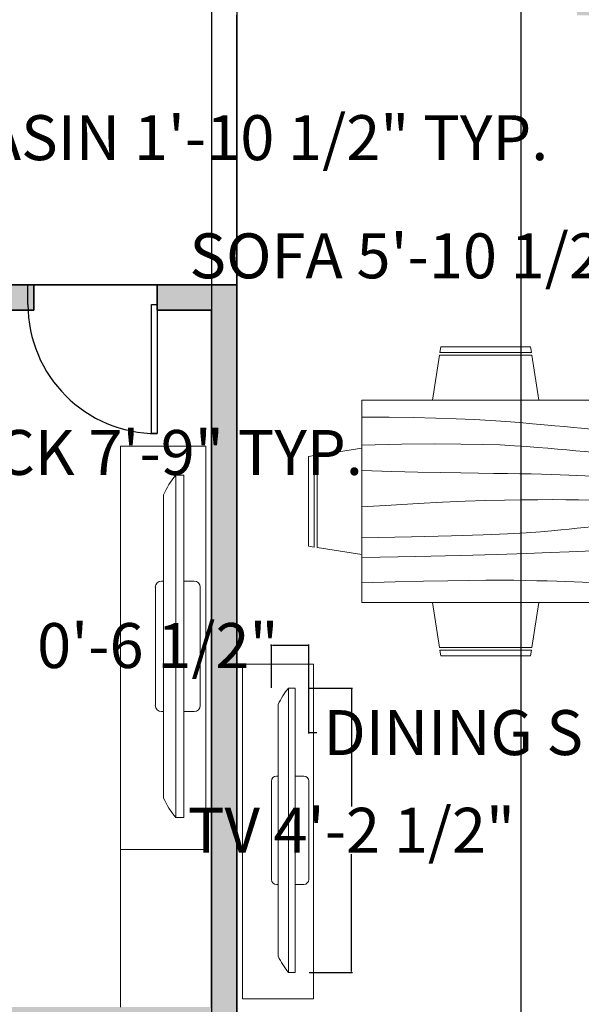
# Model space of a CAD drawing. Units: inches. Extents: x -4737294 to -4736756, y 1716389 to 1717040.
# Tile 18 of 25: x -4737096 to -4736996, y 1716669 to 1716844. Entities that reach past the tile are written whole.
import ezdxf

# ---------------------------------------------------------------- set-up
doc = ezdxf.new("R2010")
doc.units = ezdxf.units.IN
doc.header["$MEASUREMENT"] = 0
for name, color, linetype, lineweight in [('A-ANNO-DIMS', 2, 'Continuous', 18), ('A-WALL-PATT', 244, 'Continuous', 13), ('doors', 252, 'Continuous', 25), ('furniture', 250, 'Continuous', 18), ('walls', 252, 'Continuous', 35)]:
    doc.layers.add(name, color=color, linetype=linetype, lineweight=lineweight)
doc.styles.get("Standard").update_dxf_attribs({"font": 'arial.ttf'})
doc.dimstyles.get("Standard").update_dxf_attribs({"dimtxt": 8, "dimasz": 0.18, "dimexe": 0.18, "dimexo": 0.0625, "dimgap": 0.09, "dimtad": 0, "dimtih": 1, "dimtoh": 1, "dimzin": 0, "dimdsep": 46, "dimlunit": 3, "dimtxsty": 'Standard', "dimcen": 0.09, "dimadec": 0, "dimazin": 0, "dimtfac": 1, "dimtofl": 0, "dimtmove": 0, "dimatfit": 3, "dimfxl": 1, "dimtolj": 1, "dimtzin": 0, "dimarcsym": 0})

# ---------------------------------------------------------------- blocks, each defined once
blk = doc.blocks.new('Dining Set - 36 x 72 in.')
for p, q in [((-22, 27.5), (-22.1562, 26.50042)), ((-5.8416, 26.5), (-22.1534, 26.5)), ((-22, 27.5), (-6, 27.5)), ((-5.8437, 26.49966), (-6, 27.5)), ((6, 27.5), (5.8438, 26.50042)), ((22.1584, 26.5), (5.8466, 26.5)), ((6, 27.5), (22, 27.5)), ((22.1563, 26.49966), (22, 27.5)), ((-22.2343, 26.00059), (-23.4847, 17.99762)), ((-22.2304, 26), (-5.7608, 26)), ((-4.5152, 17.99762), (-5.7655, 25.99926)), ((5.7657, 26.00059), (4.5153, 17.99762)), ((5.7696, 26), (22.2392, 26)), ((23.4848, 17.99762), (22.2345, 25.99926)), ((36, 18), (-36, 18)), ((-36, 18), (-36, -18)), ((36, -18), (36, 18)), ((-44.0006, 8.23428), (-35.9976, 9.48474)), ((44.0006, 8.23428), (35.9976, 9.48474)), ((-45.5, 8), (-44.5004, 8.15617)), ((-45.5, 8), (-45.5, -8)), ((-44.5, -8.15843), (-44.5, 8.15338)), ((-44, 8.23041), (-44, -8.23915)), ((44, 8.23041), (44, -8.23915)), ((44.5, -8.15843), (44.5, 8.15338)), ((45.5, 8), (44.5005, 8.15617)), ((45.5, 8), (45.5, -8)), ((-44.4997, -8.15631), (-45.5, -8)), ((-35.9976, -9.48476), (-43.9993, -8.2345)), ((35.9976, -9.48476), (43.9993, -8.2345)), ((44.4997, -8.15631), (45.5, -8)), ((-36, -18), (36, -18)), ((-22.2343, -26.0006), (-23.4847, -17.99762)), ((-4.5152, -17.99762), (-5.7655, -25.99928)), ((5.7657, -26.0006), (4.5153, -17.99762)), ((23.4848, -17.99762), (22.2345, -25.99928)), ((-22.2304, -26), (-5.7608, -26)), ((5.7696, -26), (22.2392, -26)), ((-22, -27.5), (-22.1562, -26.50044)), ((-5.8416, -26.5), (-22.1534, -26.5)), ((-22, -27.5), (-6, -27.5)), ((-5.8437, -26.49967), (-6, -27.5)), ((6, -27.5), (5.8438, -26.50044)), ((22.1584, -26.5), (5.8466, -26.5)), ((6, -27.5), (22, -27.5)), ((22.1563, -26.49967), (22, -27.5))]:
    blk.add_line(p, q)
for points in [[(-36, 15), (-31.1772, 14.97754), (-26.8079, 14.91406), (-22.8538, 14.81543), (-19.276, 14.6875), (-16.0362, 14.53613), (-13.0957, 14.36718), (-10.4159, 14.18652), (-7.9583, 14), (-5.6904, 13.81315), (-3.6035, 13.63021), (-1.6954, 13.45508), (0.0365, 13.29166), (1.5945, 13.14388), (2.9811, 13.01562), (4.1988, 12.9108), (5.25, 12.83333), (6.1393, 12.78613), (6.8802, 12.76823), (7.4883, 12.77767), (7.9792, 12.8125), (8.3685, 12.87077), (8.6719, 12.95052), (8.9049, 13.0498), (9.0833, 13.16666), (9.2205, 13.29899), (9.3216, 13.44401), (9.3895, 13.59879), (9.4271, 13.76041), (9.4373, 13.92594), (9.4232, 14.09245), (9.3875, 14.257), (9.3333, 14.41666), (9.2638, 14.56917), (9.1836, 14.71484), (9.0975, 14.85465), (9.0104, 14.98958), (8.9272, 15.1206), (8.8529, 15.2487), (8.7922, 15.37483), (8.75, 15.5), (8.7305, 15.62467), (8.7344, 15.74739), (8.7617, 15.86621), (8.8125, 15.97916), (8.8867, 16.08431), (8.9844, 16.17968), (9.1055, 16.26334), (9.25, 16.33333), (9.4189, 16.38802), (9.6172, 16.42708), (9.8506, 16.45052), (10.125, 16.45833), (10.4463, 16.45052), (10.8203, 16.42708), (11.2529, 16.38802), (11.75, 16.33333), (12.3184, 16.26318), (12.9694, 16.17838), (13.7151, 16.07991), (14.5677, 15.96875), (15.5395, 15.84586), (16.6426, 15.71224), (17.8893, 15.56884), (19.2917, 15.41666), (20.859, 15.25667), (22.5879, 15.08984), (24.4721, 14.91715), (26.5052, 14.73958), (28.6809, 14.5581), (30.9929, 14.3737), (33.4347, 14.18733), (36, 14)], [(-36, 10), (-28.9766, 10.14274), (-23.1725, 10.20442), (-18.4241, 10.19775), (-14.5677, 10.13541), (-11.4399, 10.03011), (-8.877, 9.89453), (-6.7154, 9.74137), (-4.7917, 9.58333), (-2.9698, 9.43082), (-1.2246, 9.28515), (0.4415, 9.14534), (2.026, 9.01041), (3.5266, 8.87939), (4.9408, 8.7513), (6.266, 8.62516), (7.5, 8.5), (8.6411, 8.37549), (9.6914, 8.2539), (10.6538, 8.13818), (11.5312, 8.03125), (12.3267, 7.93603), (13.043, 7.85547), (13.6831, 7.79248), (14.25, 7.75), (14.7471, 7.7303), (15.1797, 7.73307), (15.5537, 7.75732), (15.875, 7.80208), (16.1494, 7.86637), (16.3828, 7.94922), (16.5811, 8.04964), (16.75, 8.16666), (16.8944, 8.29915), (17.0143, 8.44531), (17.1089, 8.60319), (17.1771, 8.77083), (17.218, 8.94629), (17.2305, 9.1276), (17.2137, 9.31282), (17.1667, 9.5), (17.0895, 9.6875), (16.987, 9.875), (16.8649, 10.0625), (16.7292, 10.25), (16.5856, 10.4375), (16.4401, 10.625), (16.2985, 10.8125), (16.1667, 11), (16.05, 11.18733), (15.9518, 11.3737), (15.8752, 11.5581), (15.8229, 11.73958), (15.798, 11.91715), (15.8034, 12.08984), (15.842, 12.25667), (15.9167, 12.41666), (16.0295, 12.56836), (16.1784, 12.70833), (16.3605, 12.83268), (16.5729, 12.9375), (16.8127, 13.01888), (17.0768, 13.07291), (17.3625, 13.0957), (17.6667, 13.08333), (17.9894, 13.03312), (18.3418, 12.94726), (18.7382, 12.82918), (19.1927, 12.68229), (19.7195, 12.51001), (20.3327, 12.31575), (21.0465, 12.10294), (21.875, 11.875), (22.8357, 11.63354), (23.959, 11.37304), (25.2786, 11.08618), (26.8282, 10.76562), (28.6414, 10.40405), (30.752, 9.99414), (33.1936, 9.52856), (36, 9)], [(-36, 5.5), (-30.7157, 5.3348), (-26.069, 5.20963), (-21.9946, 5.11767), (-18.4271, 5.05208), (-15.3009, 5.00602), (-12.5508, 4.97265), (-10.1112, 4.94515), (-7.9167, 4.91666), (-5.909, 4.88167), (-4.0586, 4.83984), (-2.3429, 4.79215), (-0.7396, 4.73958), (0.7739, 4.6831), (2.22, 4.6237), (3.6213, 4.56233), (5, 4.5), (6.373, 4.43782), (7.7344, 4.3776), (9.0723, 4.32129), (10.375, 4.27083), (11.6309, 4.22819), (12.8281, 4.19531), (13.9551, 4.17415), (15, 4.16666), (15.954, 4.17448), (16.819, 4.19791), (17.6001, 4.23698), (18.3021, 4.29166), (18.9299, 4.36198), (19.4883, 4.44791), (19.9823, 4.54948), (20.4167, 4.66666), (20.7969, 4.79899), (21.1302, 4.94401), (21.4245, 5.09879), (21.6875, 5.26041), (21.9271, 5.42594), (22.1511, 5.59245), (22.3672, 5.757), (22.5834, 5.91666), (22.8065, 6.06868), (23.0404, 6.21093), (23.2879, 6.34147), (23.5521, 6.45833), (23.8358, 6.55957), (24.142, 6.64323), (24.4735, 6.70735), (24.8334, 6.75), (25.2235, 6.76969), (25.642, 6.76692), (26.0858, 6.74267), (26.5521, 6.69791), (27.0379, 6.63362), (27.5404, 6.55078), (28.0565, 6.45036), (28.5834, 6.33333), (29.1242, 6.19987), (29.7071, 6.04687), (30.3661, 5.87044), (31.1354, 5.66666), (32.0493, 5.43164), (33.142, 5.16146), (34.4475, 4.85221), (36, 4.5)], [(-36, -1), (-30.7915, -0.6591), (-26.0195, -0.38216), (-21.6519, -0.16284), (-17.6563, 0.00521), (-14.0005, 0.12833), (-10.6523, 0.21289), (-7.5796, 0.26522), (-4.75, 0.29166), (-2.134, 0.29793), (0.2878, 0.28711), (2.5317, 0.26163), (4.6146, 0.22396), (6.5529, 0.17651), (8.3633, 0.12174), (10.0623, 0.06209), (11.6667, 0), (13.1899, -0.06201), (14.6341, -0.1211), (15.9982, -0.17432), (17.2813, -0.21875), (18.4823, -0.25147), (19.6003, -0.26953), (20.6343, -0.27002), (21.5834, -0.25), (22.4481, -0.20768), (23.2357, -0.14584), (23.9549, -0.06836), (24.6146, 0.02083), (25.2235, 0.11784), (25.7904, 0.21875), (26.3241, 0.31966), (26.8334, 0.41666), (27.3265, 0.50618), (27.8099, 0.58593), (28.2894, 0.65397), (28.7709, 0.70833), (29.2601, 0.74707), (29.763, 0.76823), (30.2855, 0.76985), (30.8334, 0.75), (31.4088, 0.70784), (31.9994, 0.64713), (32.589, 0.57275), (33.1615, 0.48958), (33.7008, 0.4025), (34.1908, 0.3164), (34.6153, 0.23616), (34.9584, 0.16666), (35.2099, 0.11165), (35.3848, 0.07031), (35.504, 0.04069), (35.5886, 0.02083), (35.6594, 0.00879), (35.7377, 0.0026), (35.8442, 0.00032), (36, 0)], [(-36, -6.5), (-27.1843, -6.31267), (-20.084, -6.1263), (-14.469, -5.9419), (-10.1094, -5.76042), (-6.7752, -5.58285), (-4.2363, -5.41016), (-2.2629, -5.24333), (-0.625, -5.08334), (0.8708, -4.93099), (2.2715, -4.78646), (3.5872, -4.64974), (4.8281, -4.52084), (6.0046, -4.39974), (7.127, -4.28646), (8.2053, -4.18099), (9.25, -4.08334), (10.2705, -3.99382), (11.2734, -3.91407), (12.2647, -3.84603), (13.25, -3.79167), (14.2354, -3.75293), (15.2266, -3.73177), (16.2295, -3.73015), (17.25, -3.75), (18.2912, -3.79248), (19.3451, -3.85547), (20.4009, -3.93604), (21.4479, -4.03125), (22.4754, -4.13819), (23.4727, -4.25391), (24.4289, -4.37549), (25.3334, -4.5), (26.1785, -4.62492), (26.9694, -4.74935), (27.7145, -4.87281), (28.4219, -4.99479), (29.1, -5.11483), (29.7572, -5.23242), (30.4016, -5.34709), (31.0417, -5.45834), (31.6837, -5.56437), (32.3262, -5.65821), (32.9658, -5.73153), (33.599, -5.77604), (34.2224, -5.78345), (34.8327, -5.74545), (35.4264, -5.65373), (36, -5.5)], [(-36, -10), (-26.4022, -9.81299), (-18.4675, -9.62891), (-11.9839, -9.45069), (-6.7396, -9.28125), (-2.5226, -9.12354), (0.8789, -8.98047), (3.6769, -8.85498), (6.0833, -8.75), (8.2767, -8.66765), (10.3021, -8.60677), (12.1712, -8.56543), (13.8958, -8.54167), (15.4876, -8.53353), (16.9583, -8.53907), (18.3197, -8.55632), (19.5834, -8.58334), (20.7616, -8.61841), (21.8685, -8.66081), (22.9188, -8.71004), (23.9271, -8.76563), (24.9081, -8.82707), (25.8763, -8.89388), (26.8465, -8.96558), (27.8334, -9.04167), (28.8474, -9.12118), (29.8828, -9.20117), (30.93, -9.27824), (31.9792, -9.34896), (33.0205, -9.40991), (34.0443, -9.45768), (35.0407, -9.48885), (36, -9.5)], [(-36, -14.5), (-30.0881, -14.33513), (-25.0332, -14.21224), (-20.7312, -14.12647), (-17.0781, -14.07292), (-13.97, -14.04671), (-11.3027, -14.04297), (-8.9724, -14.05681), (-6.875, -14.08334), (-4.9224, -14.11833), (-3.0905, -14.16016), (-1.3709, -14.20785), (0.2448, -14.26042), (1.7647, -14.3169), (3.1973, -14.3763), (4.5507, -14.43767), (5.8333, -14.5), (7.0554, -14.5621), (8.235, -14.62175), (9.3922, -14.67652), (10.5469, -14.72396), (11.7192, -14.76164), (12.929, -14.78711), (14.1965, -14.79794), (15.5417, -14.79167), (16.9933, -14.76424), (18.6152, -14.70508), (20.4804, -14.60197), (22.6615, -14.44271), (25.2312, -14.21509), (28.2624, -13.9069), (31.8277, -13.50594), (36, -13)]]:
    blk.add_lwpolyline(points)
blk = doc.blocks.new('PLASMA-LARGE')
at = {"layer": 'furniture'}
for p, q in [((-7.26, 0), (7.26, 0)), ((-18.61, -1), (18.61, -1)), ((-8, -1), (-8, -0.74)), ((8, -1), (8, -0.74)), ((-21, -2.5), (21, -2.5)), ((-21, -2.5), (-21, -3.5)), ((-21, -3.5), (21, -3.5)), ((-8, -3.5), (-8, -4.76)), ((8, -3.5), (8, -4.76)), ((21, -2.5), (21, -3.5)), ((-7.26, -5.5), (7.26, -5.5))]:
    blk.add_line(p, q, dxfattribs=at)
for centre, radius, start, end in [((-7.26, -0.74), 0.744, 90, 180), ((7.26, -0.74), 0.744, 0, 90), ((-13.97, -11.05), 11.07, 114.7602, 129.4175), ((13.97, -11.05), 11.07, 50.5825, 65.2398), ((-7.26, -4.76), 0.744, 180, 270), ((7.26, -4.76), 0.744, 270, 0)]:
    blk.add_arc(centre, radius, start, end, dxfattribs=at)
blk = doc.blocks.new('*U20')
for p, q in [((0, 0), (0, -6)), ((40, 0), (40, -6))]:
    blk.add_line(p, q)
blk.add_lwpolyline([(0, 0), (0, 40), (1.75, 40), (1.75, 0)], close=True)
blk.add_arc((0, 0), 40, 0, 90)
blk = doc.blocks.new('TV-CONSOLE-BEDROOM')
for p, q in [((15.21, 71.77), (0, 71.77)), ((0, 71.77), (0, 0)), ((15.21, 0), (15.21, 71.77)), ((0, 0), (15.21, 0))]:
    blk.add_line(p, q)
at = {"xscale": 1.450199298177205, "yscale": 1.450199298177205, "zscale": 1.450199298177205, "rotation": 90}
blk.add_blockref('PLASMA-LARGE', (6.22, 36.13), dxfattribs=at)
blk = doc.blocks.new('*D37')
at = {"layer": 'A-ANNO-DIMS', "color": 0, "lineweight": -2, "transparency": 16777216}
for p, q in [((-4737237.19, 1716780.66), (-4737237.19, 1716766.58)), ((-4737144.14, 1716780.66), (-4737144.14, 1716766.58)), ((-4737237.01, 1716766.76), (-4737144.32, 1716766.76)), ((-4737144.14, 1716766.76), (-4737143.96, 1716766.76))]:
    blk.add_line(p, q, dxfattribs=at)
at = {"layer": 'A-ANNO-DIMS', "color": 0, "transparency": 16777216}
for points in [[(-4737237.01, 1716766.79), (-4737237.01, 1716766.73), (-4737237.19, 1716766.76)], [(-4737144.32, 1716766.79), (-4737144.32, 1716766.73), (-4737144.14, 1716766.76)]]:
    blk.add_solid(points, dxfattribs=at)
at = {"layer": 'Defpoints', "color": 0, "transparency": 16777216}
for p in [(-4737237.19, 1716780.72), (-4737144.14, 1716780.72), (-4737144.14, 1716766.76)]:
    blk.add_point(p, dxfattribs=at)
at = {"layer": 'A-ANNO-DIMS', "color": 0, "transparency": 16777216, "insert": (-4737087.97, 1716766.76), "char_height": 8, "attachment_point": 5}
blk.add_mtext('\\A1;WC BLOCK 7\'-9" TYP.', dxfattribs=at)
blk = doc.blocks.new('*D41')
at = {"layer": 'A-ANNO-DIMS', "color": 0, "lineweight": -2, "transparency": 16777216}
for p, q in [((-4737133.94, 1716826.11), (-4737133.94, 1716822.59)), ((-4737111.26, 1716826.11), (-4737111.26, 1716822.59)), ((-4737133.76, 1716822.77), (-4737111.44, 1716822.77)), ((-4737111.26, 1716822.77), (-4737111.08, 1716822.77))]:
    blk.add_line(p, q, dxfattribs=at)
at = {"layer": 'A-ANNO-DIMS', "color": 0, "transparency": 16777216}
for points in [[(-4737133.76, 1716822.8), (-4737133.76, 1716822.74), (-4737133.94, 1716822.77)], [(-4737111.44, 1716822.8), (-4737111.44, 1716822.74), (-4737111.26, 1716822.77)]]:
    blk.add_solid(points, dxfattribs=at)
at = {"layer": 'Defpoints', "color": 0, "transparency": 16777216}
for p in [(-4737133.94, 1716826.17), (-4737111.26, 1716826.17), (-4737111.26, 1716822.77)]:
    blk.add_point(p, dxfattribs=at)
at = {"layer": 'A-ANNO-DIMS', "color": 0, "transparency": 16777216, "insert": (-4737056.03, 1716822.77), "char_height": 8, "attachment_point": 5}
blk.add_mtext('\\A1;BASIN 1\'-10 1/2" TYP.', dxfattribs=at)
blk = doc.blocks.new('*D45')
at = {"layer": 'A-ANNO-DIMS', "color": 0, "lineweight": -2, "transparency": 16777216}
for p, q in [((-4736960.53, 1716812.27), (-4736960.53, 1716801.56)), ((-4736889.92, 1716812.27), (-4736889.92, 1716801.56)), ((-4736960.53, 1716801.74), (-4736960.71, 1716801.74)), ((-4736890.1, 1716801.74), (-4736960.35, 1716801.74))]:
    blk.add_line(p, q, dxfattribs=at)
at = {"layer": 'A-ANNO-DIMS', "color": 0, "transparency": 16777216}
for points in [[(-4736960.35, 1716801.77), (-4736960.35, 1716801.71), (-4736960.53, 1716801.74)], [(-4736890.1, 1716801.77), (-4736890.1, 1716801.71), (-4736889.92, 1716801.74)]]:
    blk.add_solid(points, dxfattribs=at)
at = {"layer": 'Defpoints', "color": 0, "transparency": 16777216}
for p in [(-4736960.53, 1716812.33), (-4736889.92, 1716812.33), (-4736960.53, 1716801.74)]:
    blk.add_point(p, dxfattribs=at)
at = {"layer": 'A-ANNO-DIMS', "color": 0, "transparency": 16777216, "insert": (-4737014.36, 1716801.74), "char_height": 8, "attachment_point": 5}
blk.add_mtext('\\A1;SOFA 5\'-10 1/2" TYP.', dxfattribs=at)
blk = doc.blocks.new('*D53')
at = {"layer": 'A-ANNO-DIMS', "color": 0, "lineweight": -2, "transparency": 16777216}
for p, q in [((-4737044.89, 1716730.5), (-4737044.89, 1716716.73)), ((-4736953.89, 1716730.5), (-4736953.89, 1716716.73)), ((-4737044.71, 1716716.91), (-4737043.44, 1716716.91)), ((-4736954.07, 1716716.91), (-4736955.34, 1716716.91))]:
    blk.add_line(p, q, dxfattribs=at)
at = {"layer": 'A-ANNO-DIMS', "color": 0, "transparency": 16777216}
for points in [[(-4737044.71, 1716716.94), (-4737044.71, 1716716.88), (-4737044.89, 1716716.91)], [(-4736954.07, 1716716.94), (-4736954.07, 1716716.88), (-4736953.89, 1716716.91)]]:
    blk.add_solid(points, dxfattribs=at)
at = {"layer": 'Defpoints', "color": 0, "transparency": 16777216}
for p in [(-4737044.89, 1716730.56), (-4736953.89, 1716730.56), (-4736953.89, 1716716.91)]:
    blk.add_point(p, dxfattribs=at)
at = {"layer": 'A-ANNO-DIMS', "color": 0, "transparency": 16777216, "insert": (-4736999.39, 1716716.91), "char_height": 8, "attachment_point": 5}
blk.add_mtext('\\A1;DINING SET 7\'-7"', dxfattribs=at)
blk = doc.blocks.new('*D57')
at = {"layer": 'A-ANNO-DIMS', "color": 0, "lineweight": -2, "transparency": 16777216}
for p, q in [((-4737044.79, 1716724.81), (-4737037.09, 1716724.81)), ((-4737037.27, 1716724.63), (-4737037.27, 1716703.75)), ((-4737037.27, 1716674.42), (-4737037.27, 1716695.3)), ((-4737044.79, 1716674.24), (-4737037.09, 1716674.24))]:
    blk.add_line(p, q, dxfattribs=at)
at = {"layer": 'A-ANNO-DIMS', "color": 0, "transparency": 16777216}
for points in [[(-4737037.3, 1716724.63), (-4737037.24, 1716724.63), (-4737037.27, 1716724.81)], [(-4737037.3, 1716674.42), (-4737037.24, 1716674.42), (-4737037.27, 1716674.24)]]:
    blk.add_solid(points, dxfattribs=at)
at = {"layer": 'Defpoints', "color": 0, "transparency": 16777216}
for p in [(-4737044.86, 1716724.81), (-4737037.27, 1716724.81), (-4737044.86, 1716674.24)]:
    blk.add_point(p, dxfattribs=at)
at = {"layer": 'A-ANNO-DIMS', "color": 0, "transparency": 16777216, "insert": (-4737037.27, 1716699.53), "char_height": 8, "attachment_point": 5}
blk.add_mtext('\\A1;TV 4\'-2 1/2"', dxfattribs=at)
blk = doc.blocks.new('*D58')
at = {"layer": 'A-ANNO-DIMS', "color": 0, "lineweight": -2, "transparency": 16777216}
for p, q in [((-4737051.48, 1716732.4), (-4737051.66, 1716732.4)), ((-4737051.48, 1716724.88), (-4737051.48, 1716732.58)), ((-4737045.04, 1716732.4), (-4737051.3, 1716732.4)), ((-4737044.86, 1716724.88), (-4737044.86, 1716732.58))]:
    blk.add_line(p, q, dxfattribs=at)
at = {"layer": 'A-ANNO-DIMS', "color": 0, "transparency": 16777216}
for points in [[(-4737051.3, 1716732.43), (-4737051.3, 1716732.37), (-4737051.48, 1716732.4)], [(-4737045.04, 1716732.43), (-4737045.04, 1716732.37), (-4737044.86, 1716732.4)]]:
    blk.add_solid(points, dxfattribs=at)
at = {"layer": 'Defpoints', "color": 0, "transparency": 16777216}
for p in [(-4737051.48, 1716732.4), (-4737051.48, 1716724.81), (-4737044.86, 1716724.81)]:
    blk.add_point(p, dxfattribs=at)
at = {"layer": 'A-ANNO-DIMS', "color": 0, "transparency": 16777216, "insert": (-4737071.7, 1716732.4), "char_height": 8, "attachment_point": 5}
blk.add_mtext('\\A1;0\'-6 1/2"', dxfattribs=at)
blk = doc.blocks.new('*D62')
at = {"layer": 'A-ANNO-DIMS', "color": 0, "lineweight": -2, "transparency": 16777216}
for p, q in [((-4737062.14, 1716849), (-4737062.14, 1716423.69)), ((-4737057.64, 1716849), (-4737057.64, 1716423.69)), ((-4737061.96, 1716423.87), (-4737057.82, 1716423.87)), ((-4737057.64, 1716423.87), (-4737057.46, 1716423.87))]:
    blk.add_line(p, q, dxfattribs=at)
at = {"layer": 'A-ANNO-DIMS', "color": 0, "transparency": 16777216}
for points in [[(-4737061.96, 1716423.9), (-4737061.96, 1716423.84), (-4737062.14, 1716423.87)], [(-4737057.82, 1716423.9), (-4737057.82, 1716423.84), (-4737057.64, 1716423.87)]]:
    blk.add_solid(points, dxfattribs=at)
at = {"layer": 'Defpoints', "color": 0, "transparency": 16777216}
for p in [(-4737062.14, 1716849.06), (-4737057.64, 1716849.06), (-4737057.64, 1716423.87)]:
    blk.add_point(p, dxfattribs=at)
at = {"layer": 'A-ANNO-DIMS', "color": 0, "transparency": 16777216, "insert": (-4737037.42, 1716423.87), "char_height": 8, "attachment_point": 5}
blk.add_mtext('\\A1;0\'-4 1/2"', dxfattribs=at)
blk = doc.blocks.new('*D65')
at = {"layer": 'A-ANNO-DIMS', "color": 0, "lineweight": -2, "transparency": 16777216}
for p, q in [((-4737007.1, 1716596.13), (-4737007.1, 1717035.24)), ((-4737006.92, 1717035.06), (-4736984.27, 1717035.06)), ((-4736984.09, 1716596.13), (-4736984.09, 1717035.24)), ((-4736984.09, 1717035.06), (-4736983.91, 1717035.06))]:
    blk.add_line(p, q, dxfattribs=at)
at = {"layer": 'A-ANNO-DIMS', "color": 0, "transparency": 16777216}
for points in [[(-4737006.92, 1717035.09), (-4737006.92, 1717035.03), (-4737007.1, 1717035.06)], [(-4736984.27, 1717035.09), (-4736984.27, 1717035.03), (-4736984.09, 1717035.06)]]:
    blk.add_solid(points, dxfattribs=at)
at = {"layer": 'Defpoints', "color": 0, "transparency": 16777216}
for p in [(-4736984.09, 1717035.06), (-4737007.1, 1716596.06), (-4736984.09, 1716596.06)]:
    blk.add_point(p, dxfattribs=at)
at = {"layer": 'A-ANNO-DIMS', "color": 0, "transparency": 16777216, "insert": (-4736970.46, 1717035.06), "char_height": 8, "attachment_point": 5}
blk.add_mtext('\\A1;1\'-11"', dxfattribs=at)

msp = doc.modelspace()

# ---------------------------------------------------------------- hatches: boundary and pattern name
at = {"layer": 'A-WALL-PATT'}
h = msp.add_hatch(color=256, dxfattribs=at)
h.dxf.hatch_style = 1
h.paths.add_polyline_path([(-4737206.144, 1716844.565), (-4737110.144, 1716844.565), (-4737110.144, 1716823.907), (-4737105.644, 1716823.907), (-4737105.644, 1716844.565), (-4737098.44, 1716844.565), (-4737098.44, 1716849.065), (-4737206.144, 1716849.065), (-4737206.144, 1716993.065), (-4736864.144, 1716993.065), (-4736864.144, 1716849.065), (-4736963.275, 1716849.065), (-4736994.446, 1716849.065), (-4736997.144, 1716849.065), (-4736997.144, 1716844.565), (-4736864.144, 1716844.565), (-4736864.144, 1716668.565), (-4736934.391, 1716668.565), (-4736934.391, 1716664.065), (-4736864.144, 1716664.065), (-4736864.144, 1716462.065), (-4736855.144, 1716462.065), (-4736855.144, 1717002.065), (-4737215.144, 1717002.065), (-4737215.144, 1716462.065), (-4737206.144, 1716462.065), (-4737206.144, 1716659.065), (-4737062.144, 1716659.065), (-4737062.144, 1716647.493), (-4737057.644, 1716647.493), (-4737057.644, 1716796.565), (-4737071.812, 1716796.565), (-4737071.812, 1716792.065), (-4737070.805, 1716792.065), (-4737062.144, 1716792.065), (-4737062.144, 1716668.065), (-4737206.144, 1716668.065), (-4737206.144, 1716792.065), (-4737093.784, 1716792.065), (-4737093.784, 1716796.565), (-4737206.144, 1716796.565)])
h = msp.add_hatch(color=256, dxfattribs=at)
h.dxf.hatch_style = 1
h.paths.add_polyline_path([(-4737057.644, 1716600.884), (-4737062.144, 1716600.884), (-4737062.144, 1716534.565), (-4736933.144, 1716534.565), (-4736933.144, 1716462.065), (-4736924.144, 1716462.065), (-4736924.144, 1716543.565), (-4736973.144, 1716543.565), (-4736973.144, 1716668.565), (-4736977.644, 1716668.565), (-4736977.644, 1716543.565), (-4737057.644, 1716543.565), (-4737057.644, 1716591.565), (-4737007.073, 1716591.565), (-4737007.073, 1716596.065), (-4737057.644, 1716596.065)])
h.paths.add_polyline_path([(-4736962.872, 1716471.065), (-4737062.144, 1716471.065), (-4737062.144, 1716462.065), (-4736962.872, 1716462.065)], flags=17)
h.paths.add_polyline_path([(-4737161.883, 1716716.26), (-4737096.689, 1716716.26), (-4737096.689, 1716729.349), (-4737161.883, 1716729.349)], flags=9)
h.paths.add_polyline_path([(-4737161.912, 1716729.958), (-4737095.809, 1716729.958), (-4737095.809, 1716743.222), (-4737161.912, 1716743.222)], flags=9)
h.paths.add_polyline_path([(-4736943.842, 1716913.818), (-4736878.647, 1716913.818), (-4736878.647, 1716926.907), (-4736943.842, 1716926.907)], flags=9)
h.paths.add_polyline_path([(-4736943.871, 1716927.516), (-4736877.767, 1716927.516), (-4736877.767, 1716940.78), (-4736943.871, 1716940.78)], flags=9)
h = msp.add_hatch(color=256, dxfattribs=at)
h.dxf.hatch_style = 1
h.paths.add_polyline_path([(-4737105.644, 1716800.884), (-4737109.098, 1716800.884), (-4737110.144, 1716800.884), (-4737110.144, 1716796.565), (-4737105.644, 1716796.565)], flags=17)
h.paths.add_polyline_path([(-4736977.644, 1716596.065), (-4736984.094, 1716596.065), (-4736984.094, 1716592.614), (-4736984.094, 1716591.565), (-4736977.644, 1716591.565)], flags=17)
h.paths.add_polyline_path([(-4736919.247, 1716543.565), (-4736924.144, 1716543.565), (-4736924.144, 1716541.852), (-4736919.247, 1716541.852)], flags=17)
h.paths.add_polyline_path([(-4737063.149, 1716767.883), (-4737063.149, 1716696.117), (-4737078.363, 1716696.117), (-4737078.363, 1716767.883)], flags=0)
h.paths.add_polyline_path([(-4737067.067, 1716762.706), (-4737067.067, 1716743.853), (-4737065.246, 1716743.853, -0.4142136), (-4737064.167, 1716742.774), (-4737064.167, 1716721.73, -0.4142136), (-4737065.246, 1716720.65), (-4737067.067, 1716720.65), (-4737067.067, 1716701.798), (-4737068.518, 1716701.798, -0.0640419), (-4737070.693, 1716705.267), (-4737070.693, 1716720.65), (-4737071.064, 1716720.65, -0.4142136), (-4737072.143, 1716721.73), (-4737072.143, 1716742.774, -0.4142136), (-4737071.064, 1716743.853), (-4737070.693, 1716743.853), (-4737070.693, 1716759.237, -0.0640419), (-4737068.518, 1716762.706)], flags=0)
h.paths.add_polyline_path([(-4737129.14, 1716769.472), (-4737129.14, 1716693.886), (-4737160.657, 1716693.886), (-4737160.657, 1716701.381), (-4737189.495, 1716701.381), (-4737189.373, 1716688.681), (-4737203.937, 1716688.681), (-4737204.06, 1716701.381), (-4737204.06, 1716758.068), (-4737204.182, 1716770.768), (-4737189.618, 1716770.768), (-4737189.495, 1716758.068), (-4737160.657, 1716758.068), (-4737160.657, 1716769.472)], flags=0)
h.paths.add_polyline_path([(-4737184.679, 1716758.007), (-4737184.679, 1716747.779), (-4737192.22, 1716747.779), (-4737192.27, 1716747.71), (-4737192.27, 1716707.782), (-4737200.836, 1716707.782), (-4737200.836, 1716724.392), (-4737192.27, 1716724.392), (-4737192.27, 1716731.169), (-4737200.836, 1716731.169), (-4737200.836, 1716747.779), (-4737192.22, 1716747.779)], flags=0)
h.paths.add_polyline_path([(-4737192.212, 1716764.76, -1), (-4737201.588, 1716764.76, -1)], flags=0)
h.paths.add_polyline_path([(-4737192.089, 1716695.373, -1), (-4737201.466, 1716695.373, -1)], flags=0)
h.paths.add_polyline_path([(-4737161.883, 1716716.26), (-4737096.689, 1716716.26), (-4737096.689, 1716729.349), (-4737161.883, 1716729.349)], flags=8)
h.paths.add_polyline_path([(-4737161.912, 1716729.958), (-4737095.809, 1716729.958), (-4737095.809, 1716743.222), (-4737161.912, 1716743.222)], flags=8)

# ---------------------------------------------------------------- linework, layer by layer
at = {"layer": 'furniture'}
for p, q in [((-4737044.011, 1716729.113), (-4737056.643, 1716729.113)), ((-4737056.643, 1716729.113), (-4737056.643, 1716669.524)), ((-4737044.011, 1716669.524), (-4737044.011, 1716729.113)), ((-4737078.363, 1716696.117), (-4737078.363, 1716668.065)), ((-4737056.643, 1716669.524), (-4737044.011, 1716669.524))]:
    msp.add_line(p, q, dxfattribs=at)
at = {"layer": 'walls'}
for p, q in [((-4737057.644, 1716796.565), (-4737057.644, 1716844.565)), ((-4737206.144, 1716796.565), (-4737057.644, 1716796.565)), ((-4737093.784, 1716792.065), (-4737093.784, 1716796.565)), ((-4737071.812, 1716792.065), (-4737071.812, 1716796.565)), ((-4737057.644, 1716647.493), (-4737057.644, 1716796.565)), ((-4737206.144, 1716792.065), (-4737093.784, 1716792.065)), ((-4737071.812, 1716792.065), (-4737070.805, 1716792.065)), ((-4737070.805, 1716792.065), (-4737062.144, 1716792.065)), ((-4737062.144, 1716668.065), (-4737062.144, 1716792.065))]:
    msp.add_line(p, q, dxfattribs=at)

# ---------------------------------------------------------------- block references
at = {"layer": 'doors', "xscale": 0.5750671146789703, "yscale": 0.5750671146789703, "zscale": 0.5750671146789703, "rotation": 180}
msp.add_blockref('*U20', (-4737071.812, 1716793.114), dxfattribs=at)
at = {"layer": 'furniture'}
for name, p in [('Dining Set - 36 x 72 in.', (-4736999.39, 1716758.063)), ('TV-CONSOLE-BEDROOM', (-4737078.363, 1716696.117))]:
    msp.add_blockref(name, p, dxfattribs=at)
at = {"layer": 'furniture', "xscale": 1.204130733724425, "yscale": 1.204130733724425, "zscale": 1.204130733724425, "rotation": 90}
msp.add_blockref('PLASMA-LARGE', (-4737051.479, 1716699.528), dxfattribs=at)

# ---------------------------------------------------------------- dimensions: what is measured, and where the dimension line sits
at = {"layer": 'A-ANNO-DIMS'}
for base, p1, p2, picture, middle in [((-4736984.094, 1717035.065), (-4737007.097, 1716596.065), (-4736984.094, 1716596.065), '*D65', (-4736970.46, 1717035.065)), ((-4737057.644, 1716423.869), (-4737062.144, 1716849.065), (-4737057.644, 1716849.065), '*D62', (-4737037.421, 1716423.869))]:
    dim = msp.add_linear_dim(base=base, p1=p1, p2=p2, dimstyle='Standard', override={"dimdec": 1, "dimlfac": 1, "dimrnd": 0, "dimzin": 1, "dimdsep": 46, "dimlunit": 4, "dimfrac": 2}, dxfattribs=at)
    dim.commit()
    dim.dimension.update_dxf_attribs({"geometry": picture, "text_midpoint": middle})
for base, p1, p2, angle, text, picture, middle in [((-4737111.259, 1716822.768), (-4737133.935, 1716826.17), (-4737111.259, 1716826.17), 0, 'BASIN <> TYP.', '*D41', (-4737056.034, 1716822.768)), ((-4736960.528, 1716801.738), (-4736889.918, 1716812.329), (-4736960.528, 1716812.329), 180, 'SOFA <> TYP.', '*D45', (-4737014.356, 1716801.738)), ((-4737037.27, 1716724.815), (-4737044.856, 1716674.241), (-4737044.856, 1716724.815), 90, 'TV <>', '*D57', (-4737037.27, 1716699.528))]:
    dim = msp.add_linear_dim(base=base, p1=p1, p2=p2, angle=angle, text=text, dimstyle='Standard', override={"dimdec": 1, "dimlfac": 1, "dimrnd": 0, "dimzin": 1, "dimdsep": 46, "dimlunit": 4, "dimfrac": 2}, dxfattribs=at)
    dim.commit()
    dim.dimension.update_dxf_attribs({"geometry": picture, "text_midpoint": middle})
for base, p1, p2, text, picture, middle in [((-4737144.144, 1716766.764), (-4737237.19, 1716780.721), (-4737144.144, 1716780.721), 'WC BLOCK <> TYP.', '*D37', (-4737087.97, 1716766.764)), ((-4736953.89, 1716716.913), (-4737044.89, 1716730.563), (-4736953.89, 1716730.563), 'DINING SET <>', '*D53', (-4736999.39, 1716716.913))]:
    dim = msp.add_linear_dim(base=base, p1=p1, p2=p2, text=text, dimstyle='Standard', override={"dimdec": 1, "dimlfac": 1, "dimrnd": 0, "dimzin": 1, "dimdsep": 46, "dimlunit": 4, "dimfrac": 2}, dxfattribs=at)
    dim.commit()
    dim.dimension.update_dxf_attribs({"geometry": picture, "text_midpoint": middle})
dim = msp.add_linear_dim(base=(-4737051.479, 1716732.401), p1=(-4737044.856, 1716724.815), p2=(-4737051.479, 1716724.815), angle=180, dimstyle='Standard', override={"dimdec": 1, "dimlfac": 1, "dimrnd": 0, "dimzin": 1, "dimdsep": 46, "dimlunit": 4, "dimfrac": 2}, dxfattribs=at)
dim.commit()
dim.dimension.update_dxf_attribs({"geometry": '*D58', "text_midpoint": (-4737071.703, 1716732.401)})

doc.saveas('drawing.dxf')
